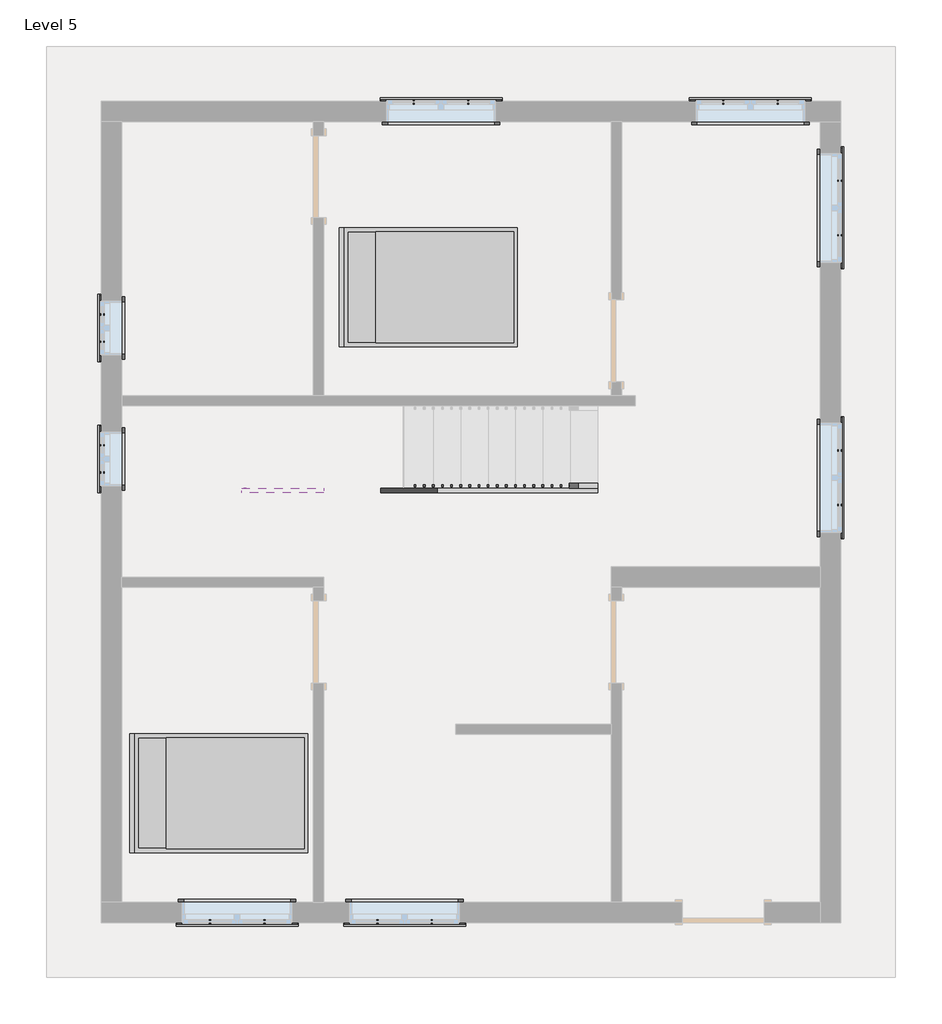
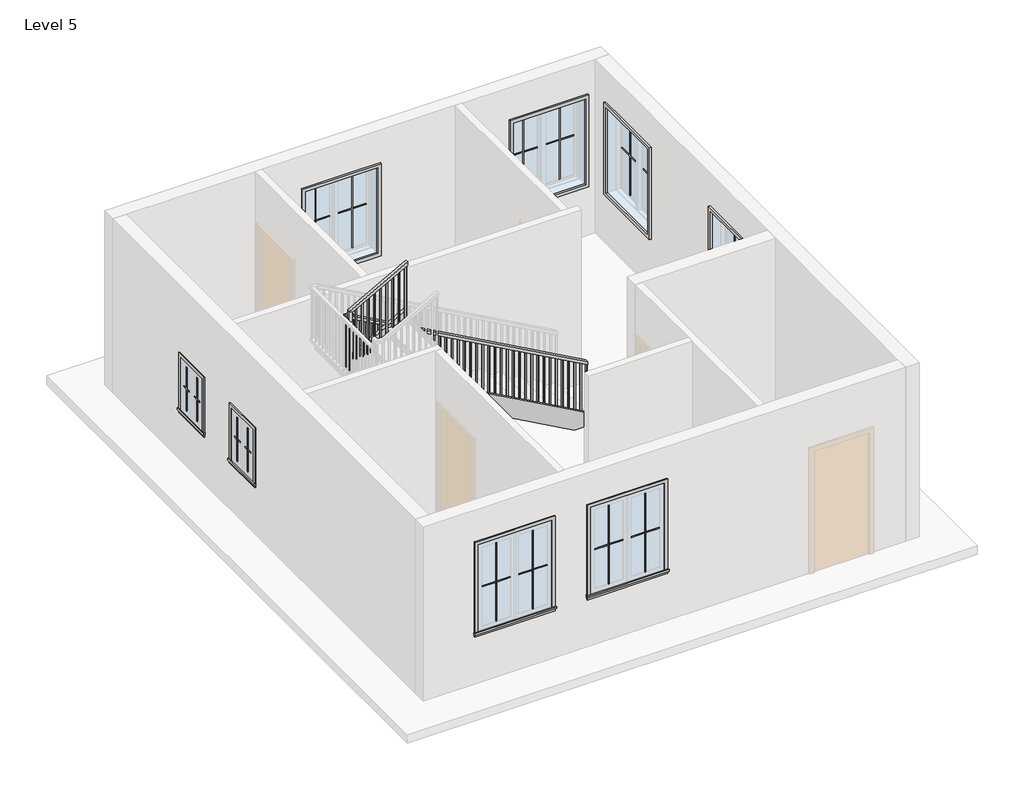
# One storey, part 2 of 2: 32 proxies, 3 members, 2 furniture elements, 1 railing.
"""IFC4 building model written with IfcOpenShell, lengths in millimetres."""

from ifc_helpers import new_model, si_unit, frame, origin, place, context, project, spatial, polyline, outline, extrude, faceted_brep, transform, mapped, element, save
from components import muntin_pattern_2x2_muntin_pattern_2x2_53152e2c, muntin_pattern_2x2_muntin_pattern_2x2_e8f3e573, muntin_pattern_2x2_muntin_pattern_2x2_6dad3731, muntin_pattern_2x2_muntin_pattern_2x2_a30a3345, trim_window_exterior_flat_with_sill_a665a915, trim_window_exterior_flat_with_sill_92b9b949, trim_window_interior_flat_picture_frame_d485c387, trim_window_interior_flat_picture_frame_3bb882cf, bed_17739_bed_17739_15c61121

model = new_model("IFC4")

# Units and contexts
model_context = context("Model", 3, world=origin())
ifc_project = project(units=[si_unit("LENGTHUNIT", "METRE", prefix="MILLI")], contexts=[model_context])

# Site, building, storey
site = spatial("IfcSite", under=ifc_project)
building = spatial("IfcBuilding", under=site)
storey = spatial("IfcBuildingStorey", under=building, Name="Level 5", Elevation=12192.0)

# Proxies
placement = place(None, origin())
muntin_pattern_2x2_muntin_pattern_2x2_shape = muntin_pattern_2x2_muntin_pattern_2x2_53152e2c(model_context)
element("IfcBuildingElementProxy", 1, Name="Muntin Pattern_2x2 : Muntin Pattern_2x2", ObjectType="Muntin Pattern_2x2 : Muntin Pattern_2x2", at=placement, inside=storey, context=model_context, shape_type="MappedRepresentation", body=[
    mapped(muntin_pattern_2x2_muntin_pattern_2x2_shape, transform((1279.525, 12101.9997886, 13176.25), x_axis=(0.0, 1.0, 0.0), y_axis=(-1.0, 0.0, 0.0), z_axis=(0.0, 0.0, 1.0))),
])
element("IfcBuildingElementProxy", 2, Name="Muntin Pattern_2x2 : Muntin Pattern_2x2", ObjectType="Muntin Pattern_2x2 : Muntin Pattern_2x2", at=placement, inside=storey, context=model_context, shape_type="MappedRepresentation", body=[
    mapped(muntin_pattern_2x2_muntin_pattern_2x2_shape, transform((1279.525, 10644.6747886, 13176.25), x_axis=(0.0, 1.0, 0.0), y_axis=(-1.0, 0.0, 0.0), z_axis=(0.0, 0.0, 1.0))),
])
muntin_pattern_2x2_muntin_pattern_2x2_2_shape = muntin_pattern_2x2_muntin_pattern_2x2_e8f3e573(model_context)
element("IfcBuildingElementProxy", 3, Name="Muntin Pattern_2x2 : Muntin Pattern_2x2", ObjectType="Muntin Pattern_2x2 : Muntin Pattern_2x2", at=placement, inside=storey, context=model_context, shape_type="MappedRepresentation", body=[
    mapped(muntin_pattern_2x2_muntin_pattern_2x2_2_shape, transform((1279.525, 12403.6247886, 13176.25), x_axis=(0.0, -1.0, 0.0), y_axis=(1.0, 0.0, 0.0), z_axis=(0.0, 0.0, 1.0))),
])
element("IfcBuildingElementProxy", 4, Name="Muntin Pattern_2x2 : Muntin Pattern_2x2", ObjectType="Muntin Pattern_2x2 : Muntin Pattern_2x2", at=placement, inside=storey, context=model_context, shape_type="MappedRepresentation", body=[
    mapped(muntin_pattern_2x2_muntin_pattern_2x2_2_shape, transform((1279.525, 10946.2997886, 13176.25), x_axis=(0.0, -1.0, 0.0), y_axis=(1.0, 0.0, 0.0), z_axis=(0.0, 0.0, 1.0))),
])
muntin_pattern_2x2_muntin_pattern_2x2_3_shape = muntin_pattern_2x2_muntin_pattern_2x2_6dad3731(model_context)
element("IfcBuildingElementProxy", 5, Name="Muntin Pattern_2x2 : Muntin Pattern_2x2", ObjectType="Muntin Pattern_2x2 : Muntin Pattern_2x2", at=placement, inside=storey, context=model_context, shape_type="MappedRepresentation", body=[
    mapped(muntin_pattern_2x2_muntin_pattern_2x2_3_shape, transform((9490.075, 13892.6997886, 13176.25), x_axis=(0.0, -1.0, 0.0), y_axis=(1.0, 0.0, 0.0), z_axis=(0.0, 0.0, 1.0))),
])
element("IfcBuildingElementProxy", 6, Name="Muntin Pattern_2x2 : Muntin Pattern_2x2", ObjectType="Muntin Pattern_2x2 : Muntin Pattern_2x2", at=placement, inside=storey, context=model_context, shape_type="MappedRepresentation", body=[
    mapped(muntin_pattern_2x2_muntin_pattern_2x2_3_shape, transform((8193.0875, 14767.4122886, 13176.25), x_axis=(1.0, 0.0, 0.0), y_axis=(0.0, 1.0, 0.0), z_axis=(0.0, 0.0, 1.0))),
])
element("IfcBuildingElementProxy", 7, Name="Muntin Pattern_2x2 : Muntin Pattern_2x2", ObjectType="Muntin Pattern_2x2 : Muntin Pattern_2x2", at=placement, inside=storey, context=model_context, shape_type="MappedRepresentation", body=[
    mapped(muntin_pattern_2x2_muntin_pattern_2x2_3_shape, transform((4749.8, 14767.4122886, 13176.25), x_axis=(1.0, 0.0, 0.0), y_axis=(0.0, 1.0, 0.0), z_axis=(0.0, 0.0, 1.0))),
])
element("IfcBuildingElementProxy", 8, Name="Muntin Pattern_2x2 : Muntin Pattern_2x2", ObjectType="Muntin Pattern_2x2 : Muntin Pattern_2x2", at=placement, inside=storey, context=model_context, shape_type="MappedRepresentation", body=[
    mapped(muntin_pattern_2x2_muntin_pattern_2x2_3_shape, transform((9490.075, 10889.1497886, 13176.25), x_axis=(0.0, -1.0, 0.0), y_axis=(1.0, 0.0, 0.0), z_axis=(0.0, 0.0, 1.0))),
])
element("IfcBuildingElementProxy", 9, Name="Muntin Pattern_2x2 : Muntin Pattern_2x2", ObjectType="Muntin Pattern_2x2 : Muntin Pattern_2x2", at=placement, inside=storey, context=model_context, shape_type="MappedRepresentation", body=[
    mapped(muntin_pattern_2x2_muntin_pattern_2x2_3_shape, transform((4950.6207347, 5642.4622886, 13176.25), x_axis=(-1.0, 0.0, 0.0), y_axis=(0.0, -1.0, 0.0), z_axis=(0.0, 0.0, 1.0))),
])
element("IfcBuildingElementProxy", 10, Name="Muntin Pattern_2x2 : Muntin Pattern_2x2", ObjectType="Muntin Pattern_2x2 : Muntin Pattern_2x2", at=placement, inside=storey, context=model_context, shape_type="MappedRepresentation", body=[
    mapped(muntin_pattern_2x2_muntin_pattern_2x2_3_shape, transform((3086.1019847, 5642.4622886, 13176.25), x_axis=(-1.0, 0.0, 0.0), y_axis=(0.0, -1.0, 0.0), z_axis=(0.0, 0.0, 1.0))),
])
muntin_pattern_2x2_muntin_pattern_2x2_4_shape = muntin_pattern_2x2_muntin_pattern_2x2_a30a3345(model_context)
element("IfcBuildingElementProxy", 11, Name="Muntin Pattern_2x2 : Muntin Pattern_2x2", ObjectType="Muntin Pattern_2x2 : Muntin Pattern_2x2", at=placement, inside=storey, context=model_context, shape_type="MappedRepresentation", body=[
    mapped(muntin_pattern_2x2_muntin_pattern_2x2_4_shape, transform((9490.075, 13286.2747886, 13176.25), x_axis=(0.0, 1.0, 0.0), y_axis=(-1.0, 0.0, 0.0), z_axis=(0.0, 0.0, 1.0))),
])
element("IfcBuildingElementProxy", 12, Name="Muntin Pattern_2x2 : Muntin Pattern_2x2", ObjectType="Muntin Pattern_2x2 : Muntin Pattern_2x2", at=placement, inside=storey, context=model_context, shape_type="MappedRepresentation", body=[
    mapped(muntin_pattern_2x2_muntin_pattern_2x2_4_shape, transform((8799.5125, 14767.4122886, 13176.25), x_axis=(-1.0, 0.0, 0.0), y_axis=(0.0, -1.0, 0.0), z_axis=(0.0, 0.0, 1.0))),
])
element("IfcBuildingElementProxy", 13, Name="Muntin Pattern_2x2 : Muntin Pattern_2x2", ObjectType="Muntin Pattern_2x2 : Muntin Pattern_2x2", at=placement, inside=storey, context=model_context, shape_type="MappedRepresentation", body=[
    mapped(muntin_pattern_2x2_muntin_pattern_2x2_4_shape, transform((5356.225, 14767.4122886, 13176.25), x_axis=(-1.0, 0.0, 0.0), y_axis=(0.0, -1.0, 0.0), z_axis=(0.0, 0.0, 1.0))),
])
element("IfcBuildingElementProxy", 14, Name="Muntin Pattern_2x2 : Muntin Pattern_2x2", ObjectType="Muntin Pattern_2x2 : Muntin Pattern_2x2", at=placement, inside=storey, context=model_context, shape_type="MappedRepresentation", body=[
    mapped(muntin_pattern_2x2_muntin_pattern_2x2_4_shape, transform((9490.075, 10282.7247886, 13176.25), x_axis=(0.0, 1.0, 0.0), y_axis=(-1.0, 0.0, 0.0), z_axis=(0.0, 0.0, 1.0))),
])
element("IfcBuildingElementProxy", 15, Name="Muntin Pattern_2x2 : Muntin Pattern_2x2", ObjectType="Muntin Pattern_2x2 : Muntin Pattern_2x2", at=placement, inside=storey, context=model_context, shape_type="MappedRepresentation", body=[
    mapped(muntin_pattern_2x2_muntin_pattern_2x2_4_shape, transform((4344.1957347, 5642.4622886, 13176.25), x_axis=(1.0, 0.0, 0.0), y_axis=(0.0, 1.0, 0.0), z_axis=(0.0, 0.0, 1.0))),
])
element("IfcBuildingElementProxy", 16, Name="Muntin Pattern_2x2 : Muntin Pattern_2x2", ObjectType="Muntin Pattern_2x2 : Muntin Pattern_2x2", at=placement, inside=storey, context=model_context, shape_type="MappedRepresentation", body=[
    mapped(muntin_pattern_2x2_muntin_pattern_2x2_4_shape, transform((2479.6769847, 5642.4622886, 13176.25), x_axis=(1.0, 0.0, 0.0), y_axis=(0.0, 1.0, 0.0), z_axis=(0.0, 0.0, 1.0))),
])
trim_window_exterior_flat_with_sill_shape = trim_window_exterior_flat_with_sill_a665a915(model_context)
element("IfcBuildingElementProxy", 17, Name="Trim-Window-Exterior-Flat : with Sill", ObjectType="Trim-Window-Exterior-Flat : with Sill", at=placement, inside=storey, context=model_context, shape_type="MappedRepresentation", body=[
    mapped(trim_window_exterior_flat_with_sill_shape, transform((1270.0, 12252.8122886, 14020.8), x_axis=(0.0, -1.0, 0.0), y_axis=(0.0, 0.0, 1.0), z_axis=(-1.0, 0.0, 0.0))),
])
element("IfcBuildingElementProxy", 18, Name="Trim-Window-Exterior-Flat : with Sill", ObjectType="Trim-Window-Exterior-Flat : with Sill", at=placement, inside=storey, context=model_context, shape_type="MappedRepresentation", body=[
    mapped(trim_window_exterior_flat_with_sill_shape, transform((1270.0, 10795.4872886, 14020.8), x_axis=(0.0, -1.0, 0.0), y_axis=(0.0, 0.0, 1.0), z_axis=(-1.0, 0.0, 0.0))),
])
trim_window_exterior_flat_with_sill_2_shape = trim_window_exterior_flat_with_sill_92b9b949(model_context)
element("IfcBuildingElementProxy", 19, Name="Trim-Window-Exterior-Flat : with Sill", ObjectType="Trim-Window-Exterior-Flat : with Sill", at=placement, inside=storey, context=model_context, shape_type="MappedRepresentation", body=[
    mapped(trim_window_exterior_flat_with_sill_2_shape, transform((9499.6, 13589.4872886, 14630.4), x_axis=(0.0, 1.0, 0.0), y_axis=(0.0, 0.0, 1.0), z_axis=(1.0, 0.0, 0.0))),
])
element("IfcBuildingElementProxy", 20, Name="Trim-Window-Exterior-Flat : with Sill", ObjectType="Trim-Window-Exterior-Flat : with Sill", at=placement, inside=storey, context=model_context, shape_type="MappedRepresentation", body=[
    mapped(trim_window_exterior_flat_with_sill_2_shape, transform((8496.3, 14776.9372886, 14630.4), x_axis=(-1.0, 0.0, 0.0), y_axis=(0.0, 0.0, 1.0), z_axis=(0.0, 1.0, 0.0))),
])
element("IfcBuildingElementProxy", 21, Name="Trim-Window-Exterior-Flat : with Sill", ObjectType="Trim-Window-Exterior-Flat : with Sill", at=placement, inside=storey, context=model_context, shape_type="MappedRepresentation", body=[
    mapped(trim_window_exterior_flat_with_sill_2_shape, transform((5053.0125, 14776.9372886, 14630.4), x_axis=(-1.0, 0.0, 0.0), y_axis=(0.0, 0.0, 1.0), z_axis=(0.0, 1.0, 0.0))),
])
element("IfcBuildingElementProxy", 22, Name="Trim-Window-Exterior-Flat : with Sill", ObjectType="Trim-Window-Exterior-Flat : with Sill", at=placement, inside=storey, context=model_context, shape_type="MappedRepresentation", body=[
    mapped(trim_window_exterior_flat_with_sill_2_shape, transform((9499.6, 10585.9372886, 14630.4), x_axis=(0.0, 1.0, 0.0), y_axis=(0.0, 0.0, 1.0), z_axis=(1.0, 0.0, 0.0))),
])
element("IfcBuildingElementProxy", 23, Name="Trim-Window-Exterior-Flat : with Sill", ObjectType="Trim-Window-Exterior-Flat : with Sill", at=placement, inside=storey, context=model_context, shape_type="MappedRepresentation", body=[
    mapped(trim_window_exterior_flat_with_sill_2_shape, transform((4647.4082347, 5632.9372886, 14630.4), x_axis=(1.0, 0.0, 0.0), y_axis=(0.0, 0.0, 1.0), z_axis=(0.0, -1.0, 0.0))),
])
element("IfcBuildingElementProxy", 24, Name="Trim-Window-Exterior-Flat : with Sill", ObjectType="Trim-Window-Exterior-Flat : with Sill", at=placement, inside=storey, context=model_context, shape_type="MappedRepresentation", body=[
    mapped(trim_window_exterior_flat_with_sill_2_shape, transform((2782.8894847, 5632.9372886, 14630.4), x_axis=(1.0, 0.0, 0.0), y_axis=(0.0, 0.0, 1.0), z_axis=(0.0, -1.0, 0.0))),
])
trim_window_interior_flat_picture_frame_shape = trim_window_interior_flat_picture_frame_d485c387(model_context)
element("IfcBuildingElementProxy", 25, Name="Trim-Window-Interior-Flat : Picture Frame", ObjectType="Trim-Window-Interior-Flat : Picture Frame", at=placement, inside=storey, context=model_context, shape_type="MappedRepresentation", body=[
    mapped(trim_window_interior_flat_picture_frame_shape, transform((1498.6, 12252.8122886, 14020.8), x_axis=(0.0, 1.0, 0.0), y_axis=(0.0, 0.0, 1.0), z_axis=(1.0, 0.0, 0.0))),
])
element("IfcBuildingElementProxy", 26, Name="Trim-Window-Interior-Flat : Picture Frame", ObjectType="Trim-Window-Interior-Flat : Picture Frame", at=placement, inside=storey, context=model_context, shape_type="MappedRepresentation", body=[
    mapped(trim_window_interior_flat_picture_frame_shape, transform((1498.6, 10795.4872886, 14020.8), x_axis=(0.0, 1.0, 0.0), y_axis=(0.0, 0.0, 1.0), z_axis=(1.0, 0.0, 0.0))),
])
trim_window_interior_flat_picture_frame_2_shape = trim_window_interior_flat_picture_frame_3bb882cf(model_context)
element("IfcBuildingElementProxy", 27, Name="Trim-Window-Interior-Flat : Picture Frame", ObjectType="Trim-Window-Interior-Flat : Picture Frame", at=placement, inside=storey, context=model_context, shape_type="MappedRepresentation", body=[
    mapped(trim_window_interior_flat_picture_frame_2_shape, transform((9271.0, 13589.4872886, 14630.4), x_axis=(0.0, -1.0, 0.0), y_axis=(0.0, 0.0, 1.0), z_axis=(-1.0, 0.0, 0.0))),
])
element("IfcBuildingElementProxy", 28, Name="Trim-Window-Interior-Flat : Picture Frame", ObjectType="Trim-Window-Interior-Flat : Picture Frame", at=placement, inside=storey, context=model_context, shape_type="MappedRepresentation", body=[
    mapped(trim_window_interior_flat_picture_frame_2_shape, transform((8496.3, 14548.3372886, 14630.4), x_axis=(1.0, 0.0, 0.0), y_axis=(0.0, 0.0, 1.0), z_axis=(0.0, -1.0, 0.0))),
])
element("IfcBuildingElementProxy", 29, Name="Trim-Window-Interior-Flat : Picture Frame", ObjectType="Trim-Window-Interior-Flat : Picture Frame", at=placement, inside=storey, context=model_context, shape_type="MappedRepresentation", body=[
    mapped(trim_window_interior_flat_picture_frame_2_shape, transform((5053.0125, 14548.3372886, 14630.4), x_axis=(1.0, 0.0, 0.0), y_axis=(0.0, 0.0, 1.0), z_axis=(0.0, -1.0, 0.0))),
])
element("IfcBuildingElementProxy", 30, Name="Trim-Window-Interior-Flat : Picture Frame", ObjectType="Trim-Window-Interior-Flat : Picture Frame", at=placement, inside=storey, context=model_context, shape_type="MappedRepresentation", body=[
    mapped(trim_window_interior_flat_picture_frame_2_shape, transform((9271.0, 10585.9372886, 14630.4), x_axis=(0.0, -1.0, 0.0), y_axis=(0.0, 0.0, 1.0), z_axis=(-1.0, 0.0, 0.0))),
])
element("IfcBuildingElementProxy", 31, Name="Trim-Window-Interior-Flat : Picture Frame", ObjectType="Trim-Window-Interior-Flat : Picture Frame", at=placement, inside=storey, context=model_context, shape_type="MappedRepresentation", body=[
    mapped(trim_window_interior_flat_picture_frame_2_shape, transform((4647.4082347, 5861.5372886, 14630.4), x_axis=(-1.0, 0.0, 0.0), y_axis=(0.0, 0.0, 1.0), z_axis=(0.0, 1.0, 0.0))),
])
element("IfcBuildingElementProxy", 32, Name="Trim-Window-Interior-Flat : Picture Frame", ObjectType="Trim-Window-Interior-Flat : Picture Frame", at=placement, inside=storey, context=model_context, shape_type="MappedRepresentation", body=[
    mapped(trim_window_interior_flat_picture_frame_2_shape, transform((2782.8894847, 5861.5372886, 14630.4), x_axis=(-1.0, 0.0, 0.0), y_axis=(0.0, 0.0, 1.0), z_axis=(0.0, 1.0, 0.0))),
])

# Furniture
bed_17739_bed_17739_shape = bed_17739_bed_17739_15c61121(model_context)
element("IfcFurniture", 33, ObjectType="Bed_17739 : Bed_17739", at=placement, inside=storey, context=model_context, shape_type="MappedRepresentation", body=[
    mapped(bed_17739_bed_17739_shape, transform((4933.95, 12706.8372886, 12192.0), x_axis=(0.0, 1.0, 0.0), y_axis=(-1.0, 0.0, 0.0), z_axis=(0.0, 0.0, 1.0))),
])
element("IfcFurniture", 34, ObjectType="Bed_17739 : Bed_17739", at=placement, inside=storey, context=model_context, shape_type="MappedRepresentation", body=[
    mapped(bed_17739_bed_17739_shape, transform((2603.5, 7074.3872886, 12192.0), x_axis=(0.0, 1.0, 0.0), y_axis=(-1.0, 0.0, 0.0), z_axis=(0.0, 0.0, 1.0))),
])

# Members
element("IfcMember", 35, ObjectType="Stringer - 2\" Width", at=placement, inside=storey, context=model_context, shape_type="SweptSolid", body=[
    extrude(outline(polyline([(12192.0, 6794.5), (12399.5983948, 6794.5), (14572.7095059, 2882.9), (14224.0308318, 2882.9), (12192.0, 6540.5554972), (12192.0, 6794.5)])), frame((0.0, 10420.8372886, 0.0), z_axis=(0.0, 1.0, 0.0), x_axis=(0.0, 0.0, 1.0)), (0.0, 0.0, 1.0), 50.8),
])
element("IfcMember", 36, ObjectType="Stringer - 2\" Width", at=placement, inside=storey, context=model_context, shape_type="SweptSolid", body=[
    extrude(outline(polyline([(2832.1, 10471.6372886), (2882.9, 10471.6372886), (2882.9, 10469.0972886), (2832.1, 10469.0972886), (2832.1, 10471.6372886)])), frame((0.0, 0.0, 14334.0666667), z_axis=(0.0, 0.0, 1.0), x_axis=(1.0, 0.0, 0.0)), (0.0, 0.0, 1.0), 304.8),
])
element("IfcMember", 37, ObjectType="Stringer - 2\" Width", at=placement, inside=storey, context=model_context, shape_type="SweptSolid", body=[
    extrude(outline(polyline([(14770.2650614, 2832.1), (14421.5863873, 2832.1), (14929.5874899, 3746.5019847), (15278.266164, 3746.5019847), (14770.2650614, 2832.1)])), frame((0.0, 10418.2972886, 0.0), z_axis=(0.0, 1.0, 0.0), x_axis=(0.0, 0.0, 1.0)), (0.0, 0.0, 1.0), 50.8),
])

# Railing
element("IfcRailing", 38, ObjectType="Handrail - Rectangular", at=placement, inside=storey, context=model_context, shape_type="SolidModel", body=[
    faceted_brep([(6794.5, 10471.6372886, 13275.7333333), (6794.5, 10471.6372886, 13217.620221), (6794.5, 10522.4372886, 13217.620221), (6794.5, 10522.4372886, 13275.7333333), (2908.3, 10471.6372886, 15434.7333333), (2857.5, 10471.6372886, 15404.8424432), (2857.5, 10522.4372886, 15404.8424432), (2908.3, 10522.4372886, 15434.7333333), (2908.3, 10471.6372886, 15477.0666667), (2857.5, 10471.6372886, 15426.2666667), (2857.5, 10522.4372886, 15426.2666667), (2908.3, 10522.4372886, 15477.0666667), (2832.1, 10471.6372886, 15477.0666667), (2832.1, 10471.6372886, 15426.2666667), (2781.3, 10522.4372886, 15426.2666667), (2781.3, 10522.4372886, 15477.0666667), (2832.1, 10395.4372886, 15477.0666667), (2832.1, 10395.4372886, 15426.2666667), (2781.3, 10395.4372886, 15426.2666667), (2781.3, 10395.4372886, 15477.0666667), (2832.1, 10392.8972886, 15477.0666667), (2781.3, 10392.8972886, 15477.0666667), (2781.3, 10392.8972886, 15426.2666667), (2832.1, 10392.8972886, 15426.2666667)], [[[0, 1, 2, 3]], [[1, 0, 4, 5]], [[2, 1, 5, 6]], [[3, 2, 6, 7]], [[0, 3, 7, 4]], [[5, 4, 8, 9]], [[6, 5, 9, 10]], [[7, 6, 10, 11]], [[4, 7, 11, 8]], [[9, 8, 12, 13]], [[10, 9, 13, 14]], [[11, 10, 14, 15]], [[8, 11, 15, 12]], [[13, 12, 16, 17]], [[14, 13, 17, 18]], [[15, 14, 18, 19]], [[12, 15, 19, 16]], [[20, 21, 22, 23]], [[17, 16, 20, 23]], [[18, 17, 23, 22]], [[19, 18, 22, 21]], [[16, 19, 21, 20]]]),
    faceted_brep([(2832.1, 10418.2972886, 15477.0666667), (2832.1, 10367.4972886, 15426.2666667), (2781.3, 10367.4972886, 15426.2666667), (2781.3, 10418.2972886, 15477.0666667), (2832.1, 10418.2972886, 15588.2869174), (2781.3, 10418.2972886, 15618.177839), (2781.3, 10367.4972886, 15618.177839), (2832.1, 10367.4972886, 15588.2869174)], [[[0, 1, 2, 3]], [[4, 5, 6, 7]], [[1, 0, 4, 7]], [[2, 1, 7, 6]], [[3, 2, 6, 5]], [[0, 3, 5, 4]]]),
    faceted_brep([(2781.3, 10418.2972886, 15618.177839), (2832.1, 10418.2972886, 15588.2869174), (2832.1, 10367.4972886, 15588.2869174), (2781.3, 10367.4972886, 15618.177839), (3746.5019847, 10418.2972886, 16154.4), (3746.5019847, 10367.4972886, 16154.4), (3746.5019847, 10367.4972886, 16096.2869174), (3746.5019847, 10418.2972886, 16096.2869174)], [[[0, 1, 2, 3]], [[4, 5, 6, 7]], [[1, 0, 4, 7]], [[2, 1, 7, 6]], [[3, 2, 6, 5]], [[0, 3, 5, 4]]]),
    extrude(outline(polyline([(16076.8838142, 3711.575), (15070.6666667, 3711.575), (15070.6666667, 3730.625), (16087.4671246, 3730.625), (16076.8838142, 3711.575)])), frame((0.0, 10383.3722886, 0.0), z_axis=(0.0, 1.0, 0.0), x_axis=(0.0, 0.0, 1.0)), (0.0, 0.0, 1.0), 19.05),
    extrude(outline(polyline([(16020.4394923, 3609.975), (15070.6666667, 3609.975), (15070.6666667, 3629.025), (16031.0228026, 3629.025), (16020.4394923, 3609.975)])), frame((0.0, 10383.3722886, 0.0), z_axis=(0.0, 1.0, 0.0), x_axis=(0.0, 0.0, 1.0)), (0.0, 0.0, 1.0), 19.05),
    extrude(outline(polyline([(15963.9951703, 3508.375), (15070.6666667, 3508.375), (15070.6666667, 3527.425), (15974.5784807, 3527.425), (15963.9951703, 3508.375)])), frame((0.0, 10383.3722886, 0.0), z_axis=(0.0, 1.0, 0.0), x_axis=(0.0, 0.0, 1.0)), (0.0, 0.0, 1.0), 19.05),
    extrude(outline(polyline([(15907.5504809, 3406.775), (14901.3333333, 3406.775), (14901.3333333, 3425.825), (15918.1337912, 3425.825), (15907.5504809, 3406.775)])), frame((0.0, 10383.3722886, 0.0), z_axis=(0.0, 1.0, 0.0), x_axis=(0.0, 0.0, 1.0)), (0.0, 0.0, 1.0), 19.05),
    extrude(outline(polyline([(15851.1061589, 3305.175), (14901.3333333, 3305.175), (14901.3333333, 3324.225), (15861.6894693, 3324.225), (15851.1061589, 3305.175)])), frame((0.0, 10383.3722886, 0.0), z_axis=(0.0, 1.0, 0.0), x_axis=(0.0, 0.0, 1.0)), (0.0, 0.0, 1.0), 19.05),
    extrude(outline(polyline([(15794.661837, 3203.575), (14901.3333333, 3203.575), (14901.3333333, 3222.625), (15805.2451474, 3222.625), (15794.661837, 3203.575)])), frame((0.0, 10383.3722886, 0.0), z_axis=(0.0, 1.0, 0.0), x_axis=(0.0, 0.0, 1.0)), (0.0, 0.0, 1.0), 19.05),
    extrude(outline(polyline([(15738.2171475, 3101.975), (14732.0, 3101.975), (14732.0, 3121.025), (15748.8004579, 3121.025), (15738.2171475, 3101.975)])), frame((0.0, 10383.3722886, 0.0), z_axis=(0.0, 1.0, 0.0), x_axis=(0.0, 0.0, 1.0)), (0.0, 0.0, 1.0), 19.05),
    extrude(outline(polyline([(15681.7728256, 3000.375), (14732.0, 3000.375), (14732.0, 3019.425), (15692.356136, 3019.425), (15681.7728256, 3000.375)])), frame((0.0, 10383.3722886, 0.0), z_axis=(0.0, 1.0, 0.0), x_axis=(0.0, 0.0, 1.0)), (0.0, 0.0, 1.0), 19.05),
    extrude(outline(polyline([(15625.3285037, 2898.775), (14732.0, 2898.775), (14732.0, 2917.825), (15635.911814, 2917.825), (15625.3285037, 2898.775)])), frame((0.0, 10383.3722886, 0.0), z_axis=(0.0, 1.0, 0.0), x_axis=(0.0, 0.0, 1.0)), (0.0, 0.0, 1.0), 19.05),
    extrude(outline(polyline([(2816.225, 10404.9622886), (2816.225, 10385.9122886), (2797.175, 10385.9122886), (2797.175, 10404.9622886), (2816.225, 10404.9622886)])), frame((0.0, 0.0, 14562.6666667), z_axis=(0.0, 0.0, 1.0), x_axis=(1.0, 0.0, 0.0)), (0.0, 0.0, 1.0), 863.6),
    extrude(outline(polyline([(2841.625, 10487.5122886), (2822.575, 10487.5122886), (2822.575, 10506.5622886), (2841.625, 10506.5622886), (2841.625, 10487.5122886)])), frame((0.0, 0.0, 14562.6666667), z_axis=(0.0, 0.0, 1.0), x_axis=(1.0, 0.0, 0.0)), (0.0, 0.0, 1.0), 863.6),
    extrude(outline(polyline([(15367.8007765, 2924.175), (14393.3333333, 2924.175), (14393.3333333, 2943.225), (15357.2174432, 2943.225), (15367.8007765, 2924.175)])), frame((0.0, 10487.5122886, 0.0), z_axis=(0.0, 1.0, 0.0), x_axis=(0.0, 0.0, 1.0)), (0.0, 0.0, 1.0), 19.05),
    extrude(outline(polyline([(15311.3563321, 3025.775), (14393.3333333, 3025.775), (14393.3333333, 3044.825), (15300.7729988, 3044.825), (15311.3563321, 3025.775)])), frame((0.0, 10487.5122886, 0.0), z_axis=(0.0, 1.0, 0.0), x_axis=(0.0, 0.0, 1.0)), (0.0, 0.0, 1.0), 19.05),
    extrude(outline(polyline([(15254.9118876, 3127.375), (14393.3333333, 3127.375), (14393.3333333, 3146.425), (15244.3285543, 3146.425), (15254.9118876, 3127.375)])), frame((0.0, 10487.5122886, 0.0), z_axis=(0.0, 1.0, 0.0), x_axis=(0.0, 0.0, 1.0)), (0.0, 0.0, 1.0), 19.05),
    extrude(outline(polyline([(15198.4674432, 3228.975), (14224.0, 3228.975), (14224.0, 3248.025), (15187.8841099, 3248.025), (15198.4674432, 3228.975)])), frame((0.0, 10487.5122886, 0.0), z_axis=(0.0, 1.0, 0.0), x_axis=(0.0, 0.0, 1.0)), (0.0, 0.0, 1.0), 19.05),
    extrude(outline(polyline([(15142.0229988, 3330.575), (14224.0, 3330.575), (14224.0, 3349.625), (15131.4396654, 3349.625), (15142.0229988, 3330.575)])), frame((0.0, 10487.5122886, 0.0), z_axis=(0.0, 1.0, 0.0), x_axis=(0.0, 0.0, 1.0)), (0.0, 0.0, 1.0), 19.05),
    extrude(outline(polyline([(15085.5785543, 3432.175), (14224.0, 3432.175), (14224.0, 3451.225), (15074.995221, 3451.225), (15085.5785543, 3432.175)])), frame((0.0, 10487.5122886, 0.0), z_axis=(0.0, 1.0, 0.0), x_axis=(0.0, 0.0, 1.0)), (0.0, 0.0, 1.0), 19.05),
    extrude(outline(polyline([(15029.1341099, 3533.775), (14054.6666667, 3533.775), (14054.6666667, 3552.825), (15018.5507765, 3552.825), (15029.1341099, 3533.775)])), frame((0.0, 10487.5122886, 0.0), z_axis=(0.0, 1.0, 0.0), x_axis=(0.0, 0.0, 1.0)), (0.0, 0.0, 1.0), 19.05),
    extrude(outline(polyline([(14972.6896654, 3635.375), (14054.6666667, 3635.375), (14054.6666667, 3654.425), (14962.1063321, 3654.425), (14972.6896654, 3635.375)])), frame((0.0, 10487.5122886, 0.0), z_axis=(0.0, 1.0, 0.0), x_axis=(0.0, 0.0, 1.0)), (0.0, 0.0, 1.0), 19.05),
    extrude(outline(polyline([(14916.245221, 3736.975), (14054.6666667, 3736.975), (14054.6666667, 3756.025), (14905.6618876, 3756.025), (14916.245221, 3736.975)])), frame((0.0, 10487.5122886, 0.0), z_axis=(0.0, 1.0, 0.0), x_axis=(0.0, 0.0, 1.0)), (0.0, 0.0, 1.0), 19.05),
    extrude(outline(polyline([(14859.8007765, 3838.575), (13885.3333333, 3838.575), (13885.3333333, 3857.625), (14849.2174432, 3857.625), (14859.8007765, 3838.575)])), frame((0.0, 10487.5122886, 0.0), z_axis=(0.0, 1.0, 0.0), x_axis=(0.0, 0.0, 1.0)), (0.0, 0.0, 1.0), 19.05),
    extrude(outline(polyline([(14803.3563321, 3940.175), (13885.3333333, 3940.175), (13885.3333333, 3959.225), (14792.7729988, 3959.225), (14803.3563321, 3940.175)])), frame((0.0, 10487.5122886, 0.0), z_axis=(0.0, 1.0, 0.0), x_axis=(0.0, 0.0, 1.0)), (0.0, 0.0, 1.0), 19.05),
    extrude(outline(polyline([(14746.9118876, 4041.775), (13885.3333333, 4041.775), (13885.3333333, 4060.825), (14736.3285543, 4060.825), (14746.9118876, 4041.775)])), frame((0.0, 10487.5122886, 0.0), z_axis=(0.0, 1.0, 0.0), x_axis=(0.0, 0.0, 1.0)), (0.0, 0.0, 1.0), 19.05),
    extrude(outline(polyline([(14690.4674432, 4143.375), (13716.0, 4143.375), (13716.0, 4162.425), (14679.8841099, 4162.425), (14690.4674432, 4143.375)])), frame((0.0, 10487.5122886, 0.0), z_axis=(0.0, 1.0, 0.0), x_axis=(0.0, 0.0, 1.0)), (0.0, 0.0, 1.0), 19.05),
    extrude(outline(polyline([(14634.0229988, 4244.975), (13716.0, 4244.975), (13716.0, 4264.025), (14623.4396654, 4264.025), (14634.0229988, 4244.975)])), frame((0.0, 10487.5122886, 0.0), z_axis=(0.0, 1.0, 0.0), x_axis=(0.0, 0.0, 1.0)), (0.0, 0.0, 1.0), 19.05),
    extrude(outline(polyline([(14577.5785543, 4346.575), (13716.0, 4346.575), (13716.0, 4365.625), (14566.995221, 4365.625), (14577.5785543, 4346.575)])), frame((0.0, 10487.5122886, 0.0), z_axis=(0.0, 1.0, 0.0), x_axis=(0.0, 0.0, 1.0)), (0.0, 0.0, 1.0), 19.05),
    extrude(outline(polyline([(14521.1341099, 4448.175), (13546.6666667, 4448.175), (13546.6666667, 4467.225), (14510.5507765, 4467.225), (14521.1341099, 4448.175)])), frame((0.0, 10487.5122886, 0.0), z_axis=(0.0, 1.0, 0.0), x_axis=(0.0, 0.0, 1.0)), (0.0, 0.0, 1.0), 19.05),
    extrude(outline(polyline([(14464.6896654, 4549.775), (13546.6666667, 4549.775), (13546.6666667, 4568.825), (14454.1063321, 4568.825), (14464.6896654, 4549.775)])), frame((0.0, 10487.5122886, 0.0), z_axis=(0.0, 1.0, 0.0), x_axis=(0.0, 0.0, 1.0)), (0.0, 0.0, 1.0), 19.05),
    extrude(outline(polyline([(14408.245221, 4651.375), (13546.6666667, 4651.375), (13546.6666667, 4670.425), (14397.6618876, 4670.425), (14408.245221, 4651.375)])), frame((0.0, 10487.5122886, 0.0), z_axis=(0.0, 1.0, 0.0), x_axis=(0.0, 0.0, 1.0)), (0.0, 0.0, 1.0), 19.05),
    extrude(outline(polyline([(14351.8007765, 4752.975), (13377.3333333, 4752.975), (13377.3333333, 4772.025), (14341.2174432, 4772.025), (14351.8007765, 4752.975)])), frame((0.0, 10487.5122886, 0.0), z_axis=(0.0, 1.0, 0.0), x_axis=(0.0, 0.0, 1.0)), (0.0, 0.0, 1.0), 19.05),
    extrude(outline(polyline([(14295.3563321, 4854.575), (13377.3333333, 4854.575), (13377.3333333, 4873.625), (14284.7729988, 4873.625), (14295.3563321, 4854.575)])), frame((0.0, 10487.5122886, 0.0), z_axis=(0.0, 1.0, 0.0), x_axis=(0.0, 0.0, 1.0)), (0.0, 0.0, 1.0), 19.05),
    extrude(outline(polyline([(14238.9118876, 4956.175), (13377.3333333, 4956.175), (13377.3333333, 4975.225), (14228.3285543, 4975.225), (14238.9118876, 4956.175)])), frame((0.0, 10487.5122886, 0.0), z_axis=(0.0, 1.0, 0.0), x_axis=(0.0, 0.0, 1.0)), (0.0, 0.0, 1.0), 19.05),
    extrude(outline(polyline([(14182.4674432, 5057.775), (13208.0, 5057.775), (13208.0, 5076.825), (14171.8841099, 5076.825), (14182.4674432, 5057.775)])), frame((0.0, 10487.5122886, 0.0), z_axis=(0.0, 1.0, 0.0), x_axis=(0.0, 0.0, 1.0)), (0.0, 0.0, 1.0), 19.05),
    extrude(outline(polyline([(14126.0229988, 5159.375), (13208.0, 5159.375), (13208.0, 5178.425), (14115.4396654, 5178.425), (14126.0229988, 5159.375)])), frame((0.0, 10487.5122886, 0.0), z_axis=(0.0, 1.0, 0.0), x_axis=(0.0, 0.0, 1.0)), (0.0, 0.0, 1.0), 19.05),
    extrude(outline(polyline([(14069.5785543, 5260.975), (13208.0, 5260.975), (13208.0, 5280.025), (14058.995221, 5280.025), (14069.5785543, 5260.975)])), frame((0.0, 10487.5122886, 0.0), z_axis=(0.0, 1.0, 0.0), x_axis=(0.0, 0.0, 1.0)), (0.0, 0.0, 1.0), 19.05),
    extrude(outline(polyline([(14013.1341099, 5362.575), (13038.6666667, 5362.575), (13038.6666667, 5381.625), (14002.5507765, 5381.625), (14013.1341099, 5362.575)])), frame((0.0, 10487.5122886, 0.0), z_axis=(0.0, 1.0, 0.0), x_axis=(0.0, 0.0, 1.0)), (0.0, 0.0, 1.0), 19.05),
    extrude(outline(polyline([(13956.6896654, 5464.175), (13038.6666667, 5464.175), (13038.6666667, 5483.225), (13946.1063321, 5483.225), (13956.6896654, 5464.175)])), frame((0.0, 10487.5122886, 0.0), z_axis=(0.0, 1.0, 0.0), x_axis=(0.0, 0.0, 1.0)), (0.0, 0.0, 1.0), 19.05),
    extrude(outline(polyline([(13900.245221, 5565.775), (13038.6666667, 5565.775), (13038.6666667, 5584.825), (13889.6618876, 5584.825), (13900.245221, 5565.775)])), frame((0.0, 10487.5122886, 0.0), z_axis=(0.0, 1.0, 0.0), x_axis=(0.0, 0.0, 1.0)), (0.0, 0.0, 1.0), 19.05),
    extrude(outline(polyline([(13843.8007765, 5667.375), (12869.3333333, 5667.375), (12869.3333333, 5686.425), (13833.2174432, 5686.425), (13843.8007765, 5667.375)])), frame((0.0, 10487.5122886, 0.0), z_axis=(0.0, 1.0, 0.0), x_axis=(0.0, 0.0, 1.0)), (0.0, 0.0, 1.0), 19.05),
    extrude(outline(polyline([(13787.3563321, 5768.975), (12869.3333333, 5768.975), (12869.3333333, 5788.025), (13776.7729988, 5788.025), (13787.3563321, 5768.975)])), frame((0.0, 10487.5122886, 0.0), z_axis=(0.0, 1.0, 0.0), x_axis=(0.0, 0.0, 1.0)), (0.0, 0.0, 1.0), 19.05),
    extrude(outline(polyline([(13730.9118876, 5870.575), (12869.3333333, 5870.575), (12869.3333333, 5889.625), (13720.3285543, 5889.625), (13730.9118876, 5870.575)])), frame((0.0, 10487.5122886, 0.0), z_axis=(0.0, 1.0, 0.0), x_axis=(0.0, 0.0, 1.0)), (0.0, 0.0, 1.0), 19.05),
    extrude(outline(polyline([(13674.4674432, 5972.175), (12700.0, 5972.175), (12700.0, 5991.225), (13663.8841099, 5991.225), (13674.4674432, 5972.175)])), frame((0.0, 10487.5122886, 0.0), z_axis=(0.0, 1.0, 0.0), x_axis=(0.0, 0.0, 1.0)), (0.0, 0.0, 1.0), 19.05),
    extrude(outline(polyline([(13618.0229988, 6073.775), (12700.0, 6073.775), (12700.0, 6092.825), (13607.4396654, 6092.825), (13618.0229988, 6073.775)])), frame((0.0, 10487.5122886, 0.0), z_axis=(0.0, 1.0, 0.0), x_axis=(0.0, 0.0, 1.0)), (0.0, 0.0, 1.0), 19.05),
    extrude(outline(polyline([(13561.5785543, 6175.375), (12700.0, 6175.375), (12700.0, 6194.425), (13550.995221, 6194.425), (13561.5785543, 6175.375)])), frame((0.0, 10487.5122886, 0.0), z_axis=(0.0, 1.0, 0.0), x_axis=(0.0, 0.0, 1.0)), (0.0, 0.0, 1.0), 19.05),
    extrude(outline(polyline([(13505.1341099, 6276.975), (12530.6666667, 6276.975), (12530.6666667, 6296.025), (13494.5507765, 6296.025), (13505.1341099, 6276.975)])), frame((0.0, 10487.5122886, 0.0), z_axis=(0.0, 1.0, 0.0), x_axis=(0.0, 0.0, 1.0)), (0.0, 0.0, 1.0), 19.05),
    extrude(outline(polyline([(13448.6896654, 6378.575), (12530.6666667, 6378.575), (12530.6666667, 6397.625), (13438.1063321, 6397.625), (13448.6896654, 6378.575)])), frame((0.0, 10487.5122886, 0.0), z_axis=(0.0, 1.0, 0.0), x_axis=(0.0, 0.0, 1.0)), (0.0, 0.0, 1.0), 19.05),
    extrude(outline(polyline([(13392.245221, 6480.175), (12530.6666667, 6480.175), (12530.6666667, 6499.225), (13381.6618876, 6499.225), (13392.245221, 6480.175)])), frame((0.0, 10487.5122886, 0.0), z_axis=(0.0, 1.0, 0.0), x_axis=(0.0, 0.0, 1.0)), (0.0, 0.0, 1.0), 19.05),
    extrude(outline(polyline([(13335.8007765, 6581.775), (12361.3333333, 6581.775), (12361.3333333, 6600.825), (13325.2174432, 6600.825), (13335.8007765, 6581.775)])), frame((0.0, 10487.5122886, 0.0), z_axis=(0.0, 1.0, 0.0), x_axis=(0.0, 0.0, 1.0)), (0.0, 0.0, 1.0), 19.05),
    extrude(outline(polyline([(13279.3563321, 6683.375), (12361.3333333, 6683.375), (12361.3333333, 6702.425), (13268.7729988, 6702.425), (13279.3563321, 6683.375)])), frame((0.0, 10487.5122886, 0.0), z_axis=(0.0, 1.0, 0.0), x_axis=(0.0, 0.0, 1.0)), (0.0, 0.0, 1.0), 19.05),
    extrude(outline(polyline([(2816.225, 10402.4222886), (2816.225, 10383.3722886), (2797.175, 10383.3722886), (2797.175, 10402.4222886), (2816.225, 10402.4222886)])), frame((0.0, 0.0, 14562.6666667), z_axis=(0.0, 0.0, 1.0), x_axis=(1.0, 0.0, 0.0)), (0.0, 0.0, 1.0), 863.6),
    extrude(outline(polyline([(2816.225, 10487.5122886), (2797.175, 10487.5122886), (2797.175, 10506.5622886), (2816.225, 10506.5622886), (2816.225, 10487.5122886)])), frame((0.0, 0.0, 14562.6666667), z_axis=(0.0, 0.0, 1.0), x_axis=(1.0, 0.0, 0.0)), (0.0, 0.0, 1.0), 863.6),
    extrude(outline(polyline([(16085.703607, 3727.4519847), (15070.6666667, 3727.4519847), (15070.6666667, 3746.5019847), (16096.2869174, 3746.5019847), (16085.703607, 3727.4519847)])), frame((0.0, 10383.3722886, 0.0), z_axis=(0.0, 1.0, 0.0), x_axis=(0.0, 0.0, 1.0)), (0.0, 0.0, 1.0), 19.05),
    extrude(outline(polyline([(13228.2035543, 6775.45), (12361.3333333, 6775.45), (12361.3333333, 6794.5), (13217.620221, 6794.5), (13228.2035543, 6775.45)])), frame((0.0, 10487.5122886, 0.0), z_axis=(0.0, 1.0, 0.0), x_axis=(0.0, 0.0, 1.0)), (0.0, 0.0, 1.0), 19.05),
])

save(model, "model.ifc")

# Revit data of these elements
# Type "Muntin Pattern_2x2 : Muntin Pattern_2x2"
#   Width [instance default] = 4' - 0"
#   Thickness = 0' - 0 1/2"
#   Height [instance default] = 4' - 0"
#   Distance = 0' - 0 3/4"
#   Interior Material [instance default] = none
#   Exterior Material [instance default] = none
#   Default Elevation = 0
# Type "Trim-Window-Exterior-Flat : with Sill"
#   Trim Width = 0' - 2 1/4"
#   Trim Thickness_Picture Frame = 0' - 1 1/4"
#   Trim Thickness_with Sill = 0' - 0 3/4"
#   Sill Thickness = 0' - 1 1/4"
#   Opening Width [instance default] = 2' - 0"
#   Opening Height [instance default] = 3' - 0"
#   Default Elevation = 4' - 0"
#   Sill = yes
#   Picture Frame = no
#   Trim Material [instance default] = none
# Type "Trim-Window-Interior-Flat : Picture Frame"
#   Trim Thickness_Picture Frame = 0' - 1 1/4"
#   Trim Width = 0' - 2 1/4"
#   Trim Thickness_with Sill = 0' - 0 3/4"
#   Sill Thickness = 0' - 1 1/4"
#   Opening Width [instance default] = 2' - 0"
#   Opening Height [instance default] = 3' - 0"
#   Default Elevation = 4' - 0"
#   Sill = no
#   Picture Frame = yes
#   Trim Material [instance default] = none
# Type "Bed_17739 : Bed_17739"
#   Default Elevation = 0
# Type "Handrail - Rectangular"
#   Assembly Code = "C2010400"
#   built-in parameter 1008612 = 0.0416667 (stored number, unit not read)
#   built-in parameter 1008611 = 0.0416667 (stored number, unit not read)
#   built-in parameter 1008609 = 0.333333 (stored number, unit not read)
#   built-in parameter 1008604 = 0.166667 (stored number, unit not read)
#   built-in parameter 1008603 = 0.166667 (stored number, unit not read)
#   Railing Height = 3' - 0"
#   built-in parameter 1008630 = 2
#   built-in parameter 1008610 = 2
#   built-in parameter 1008618 = Baluster - Square : 3/4"
# Elements 1, 2, 3, 4 (IfcBuildingElementProxy, "Muntin Pattern_2x2 : Muntin Pattern_2x2")
#   Width = 0' - 6 5/8"
#   Height = 2' - 6 1/2"
#   Interior Material = Wood - Stained
#   Exterior Material = Clad - White
#   Phase Created = New Construction
#   Materials on its faces: "Clad - White", "Wood - Stained"
# Elements 5, 6, 7, 8, 9, 10, 11, 12, 13, 14, 15, 16 (IfcBuildingElementProxy, "Muntin Pattern_2x2 : Muntin Pattern_2x2")
#   Width = 1' - 6 5/8"
#   Height = 4' - 6 1/2"
#   Interior Material = Wood - Stained
#   Exterior Material = Clad - White
#   Phase Created = New Construction
#   Materials on its faces: "Clad - White", "Wood - Stained"
# Elements 17, 18 (IfcBuildingElementProxy, "Trim-Window-Exterior-Flat : with Sill")
#   Opening Width = 2' - 0"
#   Opening Height = 3' - 0"
#   Trim Material = Clad - White
#   Phase Created = New Construction
#   Materials on its faces: "Clad - White"
# Elements 19, 20, 21, 22, 23, 24 (IfcBuildingElementProxy, "Trim-Window-Exterior-Flat : with Sill")
#   Opening Width = 4' - 0"
#   Opening Height = 5' - 0"
#   Trim Material = Clad - White
#   Phase Created = New Construction
#   Materials on its faces: "Clad - White"
# Elements 25, 26 (IfcBuildingElementProxy, "Trim-Window-Interior-Flat : Picture Frame")
#   Opening Width = 2' - 0"
#   Opening Height = 3' - 0"
#   Trim Material = Wood - Stained
#   Phase Created = New Construction
#   Materials on its faces: "Wood - Stained"
# Elements 27, 28, 29, 30, 31, 32 (IfcBuildingElementProxy, "Trim-Window-Interior-Flat : Picture Frame")
#   Opening Width = 4' - 0"
#   Opening Height = 5' - 0"
#   Trim Material = Wood - Stained
#   Phase Created = New Construction
#   Materials on its faces: "Wood - Stained"
# Elements 33, 34 (IfcFurniture, "Bed_17739 : Bed_17739")
#   Phase Created = New Construction
#   Materials on its faces: "legs", "sheets", "bed frame", "Blanket"
# Elements 35, 36, 37 (IfcMember, "Stringer - 2\" Width")
#   Phase Created = New Construction
# Element 38 (IfcRailing, "Handrail - Rectangular")
#   Phase Created = New Construction
# Materials
#   "Clad - White": class "Wood", colour RGB 242 242 238, transparency 0, Cost = 0
#   "Wood - Stained": class "Wood", colour RGB 224 178 126, transparency 0, Cost = 0
#   "legs": colour RGB 90 73 37, transparency 0, Cost = 0
#   "sheets": colour RGB 200 195 176, transparency 0, Cost = 0
#   "bed frame": colour RGB 90 73 37, transparency 0, Cost = 0
#   "Blanket": class "System", colour RGB 59 0 1, transparency 0, Cost = 0
